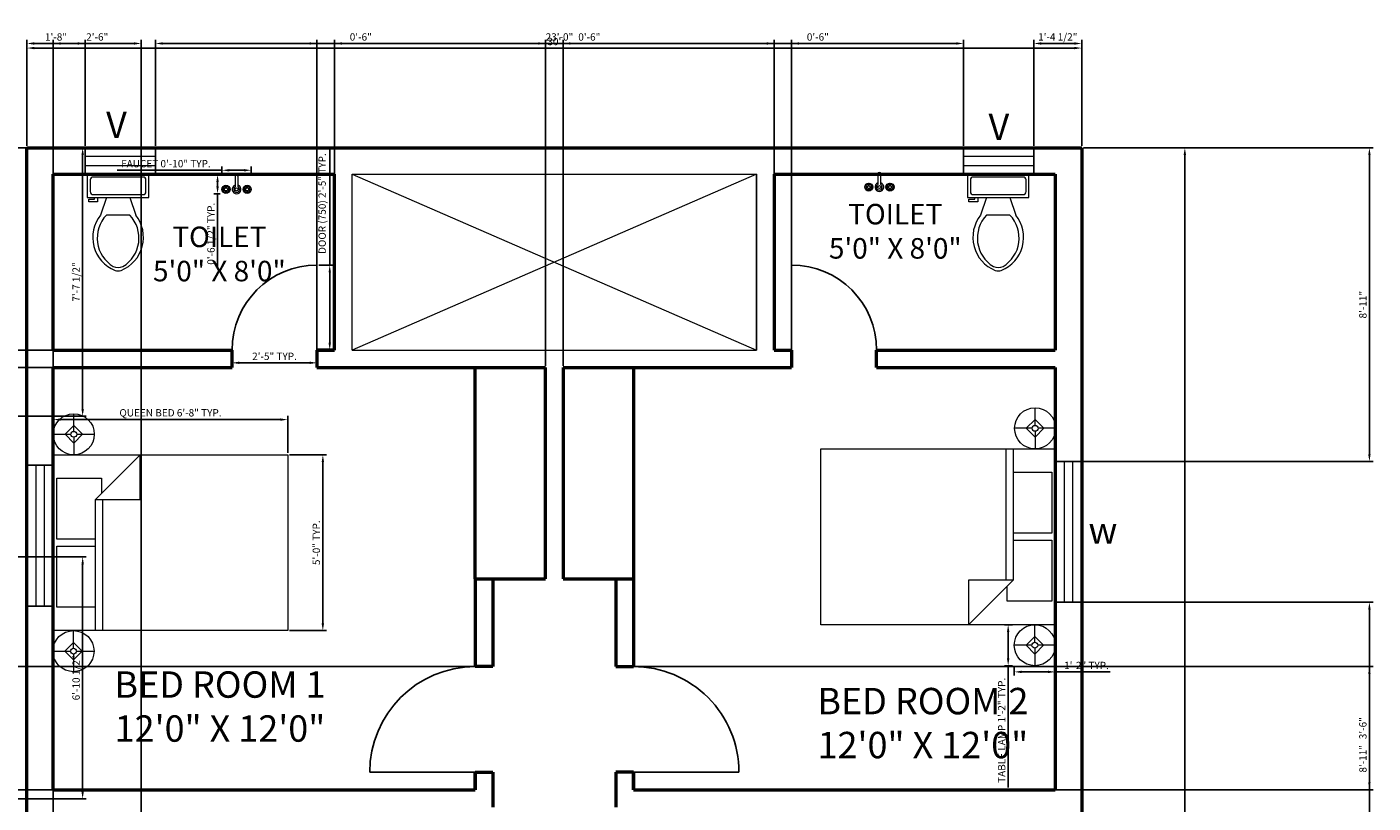
# Model space of a CAD drawing. Units: inches. Extents: x 3688 to 4628, y 1593 to 2337.
# Tile 7 of 7: x 4168 to 4628, y 2072 to 2337. Entities that reach past the tile are written whole.
import ezdxf

# ---------------------------------------------------------------- set-up
doc = ezdxf.new("R2010")
doc.units = ezdxf.units.IN
for name, color, linetype, lineweight in [('A-ANNO-DIMS', 2, 'Continuous', 18), ('A-ANNO-TEXT', 7, 'Continuous', 18), ('A-AREA-IDEN', 7, 'Continuous', 25), ('A-DOOR', 4, 'Continuous', 25), ('A-FLOR-FIXT', 8, 'Continuous', 18), ('A-FLOR-SHFT', 8, 'Continuous', 18), ('A-FURN', 8, 'Continuous', 18), ('A-GLAZ', 4, 'Continuous', 25), ('A-WALL', 7, 'Continuous', 50)]:
    doc.layers.add(name, color=color, linetype=linetype, lineweight=lineweight)
doc.styles.get("Standard").update_dxf_attribs({"font": 'arial.ttf'})
doc.dimstyles.new('ISO-25', dxfattribs={"dimtxt": 2.5, "dimasz": 2.5, "dimexe": 1.25, "dimexo": 0.625, "dimtad": 1, "dimdec": 0, "dimlunit": 3, "dimtxsty": 'Standard', "dimcen": 2.5, "dimadec": 0, "dimazin": 0, "dimtfac": 1, "dimtdec": 0, "dimtmove": 0, "dimatfit": 3, "dimfxl": 1, "dimarcsym": 0})

# ---------------------------------------------------------------- blocks, each defined once
blk = doc.blocks.new('Bed - Queen')
for p, q in [((0, -80.00003), (0, 0)), ((0, 0), (59.99999, 0)), ((59.99999, 0), (59.99999, -80.00003)), ((7.99999, -1.2), (28.79998, -1.2)), ((7.99999, -14.4), (7.99999, -1.2)), ((28.79998, -1.2), (28.79998, -14.4)), ((31.19999, -1.2), (51.99999, -1.2)), ((31.19999, -14.4), (31.19999, -1.2)), ((51.99999, -1.2), (51.99999, -16.4)), ((0, -14.4), (44.8, -14.4)), ((44.8, -16.8), (0, -16.8)), ((59.99999, -29.6), (44.8, -14.4)), ((44.8, -14.4), (44.8, -29.6)), ((51.99999, -16.4), (46.79936, -16.4)), ((44.8, -29.6), (59.99999, -29.6)), ((59.99999, -80.00003), (0, -80.00003))]:
    blk.add_line(p, q)
blk = doc.blocks.new('Lamp - Table')
for p, q in [((0, 7), (0, 1)), ((-1, 0), (-7, 0)), ((0, 3), (-3, 0)), ((-3, 0), (0, -3)), ((3, 0), (0, 3)), ((0, -3), (3, 0)), ((1, 0), (7, 0)), ((0, -1), (0, -7))]:
    blk.add_line(p, q)
for radius in [7, 1]:
    blk.add_circle((0, 0), radius)
blk = doc.blocks.new('Toilet - top')
for p, q in [((9.5, -6), (9.5, -2)), ((-10, -8.5), (-8, -8.5)), ((-10, -9.5), (-10, -8.5)), ((-8, -8.5), (-8, -8)), ((-7, -8), (-7, -9.5)), ((-4, -8), (-6, -14)), ((4, -8), (6, -14)), ((-7, -9.5), (-10, -9.5)), ((4, -14), (-4, -14))]:
    blk.add_line(p, q)
blk.add_lwpolyline([(10.5, -8), (10.5, 0), (-10.5, 0), (-10.5, -8)], close=True)
for points in [[(-9.5, -2), (-9.5, -6)], [(8.5, -1), (-8.5, -1)], [(-8.5, -7), (8.5, -7)]]:
    blk.add_lwpolyline(points)
for centre, radius, start, end in [((-8.62, -1.88), 0.884, 81.8699, 188.1301), ((8.62, -1.88), 0.884, 351.8699, 98.1301), ((-8.62, -6.12), 0.884, 171.8699, 278.1301), ((8.62, -6.12), 0.884, 261.8699, 8.1301), ((3.52, -21.58), 12.17, 141.4691, 247.9714), ((4.2, -21.82), 11.33, 136.3677, 238.9468), ((-3.52, -21.58), 12.17, 292.0284, 38.5307), ((-4.2, -21.82), 11.33, 301.053, 43.6321), ((0, -27.88), 4, 245.7318, 294.2682), ((0, -29), 4, 254.8605, 285.1395)]:
    blk.add_arc(centre, radius, start, end)
blk = doc.blocks.new('Faucet - Bathroom top')
for p, q in [((-4.107, 0.125), (-4.375, 0.125)), ((-3.75, 0.4788), (-3.75, 0.75)), ((-3.5, 0.482), (-3.5, 0.75)), ((-3.1461, 0.125), (-2.875, 0.125)), ((3.143, 0.125), (2.875, 0.125)), ((3.5, 0.4788), (3.5, 0.75)), ((3.75, 0.482), (3.75, 0.75)), ((4.1039, 0.125), (4.375, 0.125)), ((-4.1039, -0.125), (-4.375, -0.125)), ((-3.75, -0.4821), (-3.75, -0.75)), ((-3.5, -0.4789), (-3.5, -0.75)), ((-3.143, -0.125), (-2.875, -0.125)), ((-0.5, -0.8639), (-0.5, -4.5)), ((0.5, -4.5), (0.5, -0.8631)), ((3.1461, -0.125), (2.875, -0.125)), ((3.5, -0.4821), (3.5, -0.75)), ((3.75, -0.4789), (3.75, -0.75)), ((4.107, -0.125), (4.375, -0.125))]:
    blk.add_line(p, q)
for centre, radius in [((-3.625, 0), 1.375), ((-4.625, 0), 0.2795), ((-3.625, 0), 0.5), ((-3.625, 1), 0.2795), ((-2.625, 0), 0.2795), ((0, 0), 0.5), ((3.625, 0), 1.375), ((2.625, 0), 0.2795), ((3.625, 0), 0.5), ((3.625, 1), 0.2795), ((4.625, 0), 0.2795), ((-3.625, -1), 0.2795), ((3.625, -1), 0.2795)]:
    blk.add_circle(centre, radius)
for centre, radius, start, end in [((-3.625, 0), 1, 105.2407, 164.2093), ((-3.625, 0), 1, 16.44125, 74.07887), ((0, 0), 1.5, 289.6514, 250.3603), ((0, 0), 1, 300.3431, 239.7554), ((3.625, 0), 1, 106.12, 164.0884), ((3.625, 0), 1, 16.23422, 73.90469), ((-3.625, 0), 1, 196.2342, 253.9047), ((-3.625, 0), 1, 286.12, 344.0884), ((0, -4.5), 0.5, 180, 0), ((3.625, 0), 1, 196.4413, 254.0789), ((3.625, 0), 1, 285.2407, 344.2093)]:
    blk.add_arc(centre, radius, start, end)
blk = doc.blocks.new('*D14')
at = {"layer": 'A-ANNO-DIMS', "color": 0, "lineweight": -2, "transparency": 16777216}
for p, q in [((4168.13, 2295.91), (4168.13, 2330.57)), ((4528.13, 2295.91), (4528.13, 2330.57)), ((4170.63, 2329.32), (4525.63, 2329.32))]:
    blk.add_line(p, q, dxfattribs=at)
at = {"layer": 'A-ANNO-DIMS', "color": 0, "transparency": 16777216}
for points in [[(4170.63, 2329.74), (4170.63, 2328.91), (4168.13, 2329.32)], [(4525.63, 2329.74), (4525.63, 2328.91), (4528.13, 2329.32)]]:
    blk.add_solid(points, dxfattribs=at)
at = {"layer": 'Defpoints', "color": 0, "transparency": 16777216}
for p in [(4528.13, 2329.32), (4168.13, 2295.28), (4528.13, 2295.28)]:
    blk.add_point(p, dxfattribs=at)
at = {"layer": 'A-ANNO-DIMS', "color": 0, "transparency": 16777216, "insert": (4348.13, 2331.23), "char_height": 2.5, "attachment_point": 5}
blk.add_mtext("30'", dxfattribs=at)
blk = doc.blocks.new('*D15')
at = {"layer": 'A-ANNO-DIMS', "color": 0, "lineweight": -2, "transparency": 16777216}
for p, q in [((4528.76, 2295.28), (4564.58, 2295.28)), ((4563.33, 2292.78), (4563.33, 1697.78)), ((4528.76, 1695.28), (4564.58, 1695.28))]:
    blk.add_line(p, q, dxfattribs=at)
at = {"layer": 'A-ANNO-DIMS', "color": 0, "transparency": 16777216}
for points in [[(4562.91, 2292.78), (4563.75, 2292.78), (4563.33, 2295.28)], [(4562.91, 1697.78), (4563.75, 1697.78), (4563.33, 1695.28)]]:
    blk.add_solid(points, dxfattribs=at)
at = {"layer": 'Defpoints', "color": 0, "transparency": 16777216}
for p in [(4528.13, 2295.28), (4528.13, 1695.28), (4563.33, 1695.28)]:
    blk.add_point(p, dxfattribs=at)
at = {"layer": 'A-ANNO-DIMS', "color": 0, "transparency": 16777216, "insert": (4561.43, 1995.28), "char_height": 2.5, "attachment_point": 5, "rotation": 90}
blk.add_mtext("50'", dxfattribs=at)
blk = doc.blocks.new('DOOR-900')
blk.add_line((0, 0), (0, 36))
blk.add_arc((0, 0), 36, 0, 90)
blk = doc.blocks.new('DOOR-750')
blk.add_line((29, 0), (29, 29))
blk.add_arc((29, 0), 29, 90, 180)
blk = doc.blocks.new('WIN-1200')
for p, q in [((0, 48), (0, 0)), ((9, 48), (0, 48)), ((9, 0), (9, 48)), ((0, 0), (9, 0))]:
    blk.add_line(p, q)
blk = doc.blocks.new('WIN-600')
for p, q in [((24, 9), (0, 9)), ((0, 9), (0, 0)), ((24, 0), (24, 9)), ((0, 0), (24, 0))]:
    blk.add_line(p, q)
blk = doc.blocks.new('*D31')
at = {"layer": 'A-ANNO-DIMS', "color": 0, "lineweight": -2, "transparency": 16777216}
for p, q in [((4271.48, 2255.28), (4271.48, 2294.72)), ((4267.76, 2255.28), (4272.73, 2255.28)), ((4271.48, 2228.78), (4271.48, 2252.78)), ((4267.76, 2226.28), (4272.73, 2226.28))]:
    blk.add_line(p, q, dxfattribs=at)
at = {"layer": 'A-ANNO-DIMS', "color": 0, "transparency": 16777216}
for points in [[(4271.07, 2252.78), (4271.9, 2252.78), (4271.48, 2255.28)], [(4271.07, 2228.78), (4271.9, 2228.78), (4271.48, 2226.28)]]:
    blk.add_solid(points, dxfattribs=at)
at = {"layer": 'Defpoints', "color": 0, "transparency": 16777216}
for p in [(4267.13, 2255.28), (4271.48, 2255.28), (4267.13, 2226.28)]:
    blk.add_point(p, dxfattribs=at)
at = {"layer": 'A-ANNO-DIMS', "color": 0, "transparency": 16777216, "insert": (4269.22, 2276.25), "char_height": 2.5, "attachment_point": 5, "rotation": 90}
blk.add_mtext('DOOR (750) 2\'-5" TYP.', dxfattribs=at)
blk = doc.blocks.new('*D32')
at = {"layer": 'A-ANNO-DIMS', "color": 0, "lineweight": -2, "transparency": 16777216}
for p, q in [((4238.13, 2225.66), (4238.13, 2220.68)), ((4267.13, 2225.66), (4267.13, 2220.68)), ((4240.63, 2221.93), (4264.63, 2221.93))]:
    blk.add_line(p, q, dxfattribs=at)
at = {"layer": 'A-ANNO-DIMS', "color": 0, "transparency": 16777216}
for points in [[(4240.63, 2222.35), (4240.63, 2221.52), (4238.13, 2221.93)], [(4264.63, 2222.35), (4264.63, 2221.52), (4267.13, 2221.93)]]:
    blk.add_solid(points, dxfattribs=at)
at = {"layer": 'Defpoints', "color": 0, "transparency": 16777216}
for p in [(4238.13, 2226.28), (4267.13, 2226.28), (4267.13, 2221.93)]:
    blk.add_point(p, dxfattribs=at)
at = {"layer": 'A-ANNO-DIMS', "color": 0, "transparency": 16777216, "insert": (4252.63, 2223.83), "char_height": 2.5, "attachment_point": 5}
blk.add_mtext('2\'-5" TYP.', dxfattribs=at)
blk = doc.blocks.new('*D33')
at = {"layer": 'A-ANNO-DIMS', "color": 0, "lineweight": -2, "transparency": 16777216}
for p, q in [((4177.13, 2191.18), (4177.13, 2203.8)), ((4254.63, 2202.55), (4179.63, 2202.55)), ((4257.13, 2191.18), (4257.13, 2203.8))]:
    blk.add_line(p, q, dxfattribs=at)
at = {"layer": 'A-ANNO-DIMS', "color": 0, "transparency": 16777216}
for points in [[(4179.63, 2202.97), (4179.63, 2202.14), (4177.13, 2202.55)], [(4254.63, 2202.97), (4254.63, 2202.14), (4257.13, 2202.55)]]:
    blk.add_solid(points, dxfattribs=at)
at = {"layer": 'Defpoints', "color": 0, "transparency": 16777216}
for p in [(4177.13, 2202.55), (4177.13, 2190.55), (4257.13, 2190.55)]:
    blk.add_point(p, dxfattribs=at)
at = {"layer": 'A-ANNO-DIMS', "color": 0, "transparency": 16777216, "insert": (4217.13, 2204.55), "char_height": 2.5, "attachment_point": 5}
blk.add_mtext('QUEEN BED 6\'-8" TYP.', dxfattribs=at)
blk = doc.blocks.new('*D34')
at = {"layer": 'A-ANNO-DIMS', "color": 0, "lineweight": -2, "transparency": 16777216}
for p, q in [((4257.76, 2190.55), (4270.38, 2190.55)), ((4269.13, 2133.05), (4269.13, 2188.05)), ((4257.76, 2130.55), (4270.38, 2130.55))]:
    blk.add_line(p, q, dxfattribs=at)
at = {"layer": 'A-ANNO-DIMS', "color": 0, "transparency": 16777216}
for points in [[(4268.72, 2188.05), (4269.55, 2188.05), (4269.13, 2190.55)], [(4268.72, 2133.05), (4269.55, 2133.05), (4269.13, 2130.55)]]:
    blk.add_solid(points, dxfattribs=at)
at = {"layer": 'Defpoints', "color": 0, "transparency": 16777216}
for p in [(4257.13, 2190.55), (4269.13, 2190.55), (4257.13, 2130.55)]:
    blk.add_point(p, dxfattribs=at)
at = {"layer": 'A-ANNO-DIMS', "color": 0, "transparency": 16777216, "insert": (4267.23, 2160.55), "char_height": 2.5, "attachment_point": 5, "rotation": 90}
blk.add_mtext('5\'-0" TYP.', dxfattribs=at)
blk = doc.blocks.new('*D35')
at = {"layer": 'A-ANNO-DIMS', "color": 0, "lineweight": -2, "transparency": 16777216}
for p, q in [((4504.51, 2132.58), (4501.78, 2132.58)), ((4503.03, 2130.08), (4503.03, 2121.08)), ((4504.51, 2118.58), (4501.78, 2118.58)), ((4503.03, 2118.58), (4503.03, 2077.01))]:
    blk.add_line(p, q, dxfattribs=at)
at = {"layer": 'A-ANNO-DIMS', "color": 0, "transparency": 16777216}
for points in [[(4502.62, 2130.08), (4503.45, 2130.08), (4503.03, 2132.58)], [(4502.62, 2121.08), (4503.45, 2121.08), (4503.03, 2118.58)]]:
    blk.add_solid(points, dxfattribs=at)
at = {"layer": 'Defpoints', "color": 0, "transparency": 16777216}
for p in [(4505.13, 2132.58), (4503.03, 2118.58), (4505.13, 2118.58)]:
    blk.add_point(p, dxfattribs=at)
at = {"layer": 'A-ANNO-DIMS', "color": 0, "transparency": 16777216, "insert": (4501.15, 2096.55), "char_height": 2.5, "attachment_point": 5, "rotation": 90}
blk.add_mtext('TABLE LAMP 1\'-2" TYP.', dxfattribs=at)
blk = doc.blocks.new('*D36')
at = {"layer": 'A-ANNO-DIMS', "color": 0, "lineweight": -2, "transparency": 16777216}
for p, q in [((4505.13, 2117.96), (4505.13, 2115.23)), ((4507.63, 2116.48), (4516.63, 2116.48)), ((4519.13, 2117.96), (4519.13, 2115.23)), ((4519.13, 2116.48), (4537.89, 2116.48))]:
    blk.add_line(p, q, dxfattribs=at)
at = {"layer": 'A-ANNO-DIMS', "color": 0, "transparency": 16777216}
for points in [[(4507.63, 2116.9), (4507.63, 2116.07), (4505.13, 2116.48)], [(4516.63, 2116.9), (4516.63, 2116.07), (4519.13, 2116.48)]]:
    blk.add_solid(points, dxfattribs=at)
at = {"layer": 'Defpoints', "color": 0, "transparency": 16777216}
for p in [(4505.13, 2118.58), (4519.13, 2118.58), (4519.13, 2116.48)]:
    blk.add_point(p, dxfattribs=at)
at = {"layer": 'A-ANNO-DIMS', "color": 0, "transparency": 16777216, "insert": (4529.76, 2118.36), "char_height": 2.5, "attachment_point": 5}
blk.add_mtext('1\'-2" TYP.', dxfattribs=at)
blk = doc.blocks.new('*D39')
at = {"layer": 'A-ANNO-DIMS', "color": 0, "lineweight": -2, "transparency": 16777216}
for p, q in [((4234.7, 2286.75), (4234.7, 2288.88)), ((4244.7, 2286.75), (4244.7, 2288.88)), ((4234.7, 2287.63), (4198.97, 2287.63)), ((4242.2, 2287.63), (4237.2, 2287.63))]:
    blk.add_line(p, q, dxfattribs=at)
at = {"layer": 'A-ANNO-DIMS', "color": 0, "transparency": 16777216}
for points in [[(4237.2, 2288.04), (4237.2, 2287.21), (4234.7, 2287.63)], [(4242.2, 2288.04), (4242.2, 2287.21), (4244.7, 2287.63)]]:
    blk.add_solid(points, dxfattribs=at)
at = {"layer": 'Defpoints', "color": 0, "transparency": 16777216}
for p in [(4234.7, 2287.63), (4234.7, 2286.13), (4244.7, 2286.13)]:
    blk.add_point(p, dxfattribs=at)
at = {"layer": 'A-ANNO-DIMS', "color": 0, "transparency": 16777216, "insert": (4215.58, 2289.54), "char_height": 2.5, "attachment_point": 5}
blk.add_mtext('FAUCET 0\'-10" TYP.', dxfattribs=at)
blk = doc.blocks.new('*D40')
at = {"layer": 'A-ANNO-DIMS', "color": 0, "lineweight": -2, "transparency": 16777216}
for p, q in [((4234.07, 2286.13), (4231.95, 2286.13)), ((4233.2, 2283.63), (4233.2, 2282.13)), ((4234.07, 2279.63), (4231.95, 2279.63)), ((4233.2, 2279.63), (4233.2, 2254.81))]:
    blk.add_line(p, q, dxfattribs=at)
at = {"layer": 'A-ANNO-DIMS', "color": 0, "transparency": 16777216}
for points in [[(4232.78, 2283.63), (4233.61, 2283.63), (4233.2, 2286.13)], [(4232.78, 2282.13), (4233.61, 2282.13), (4233.2, 2279.63)]]:
    blk.add_solid(points, dxfattribs=at)
at = {"layer": 'Defpoints', "color": 0, "transparency": 16777216}
for p in [(4234.7, 2286.13), (4233.2, 2279.63), (4234.7, 2279.63)]:
    blk.add_point(p, dxfattribs=at)
at = {"layer": 'A-ANNO-DIMS', "color": 0, "transparency": 16777216, "insert": (4231.28, 2265.97), "char_height": 2.5, "attachment_point": 5, "rotation": 90}
blk.add_mtext('0\'-6 1/2" TYP.', dxfattribs=at)
blk = doc.blocks.new('*D57')
at = {"layer": 'A-ANNO-DIMS', "color": 0, "lineweight": -2, "transparency": 16777216}
for p, q in [((4090.25, 2295.32), (4188.4, 2295.32)), ((4187.15, 2292.82), (4187.15, 2206.19)), ((4090.25, 2203.69), (4188.4, 2203.69))]:
    blk.add_line(p, q, dxfattribs=at)
at = {"layer": 'A-ANNO-DIMS', "color": 0, "transparency": 16777216}
for points in [[(4186.74, 2292.82), (4187.57, 2292.82), (4187.15, 2295.32)], [(4186.74, 2206.19), (4187.57, 2206.19), (4187.15, 2203.69)]]:
    blk.add_solid(points, dxfattribs=at)
at = {"layer": 'Defpoints', "color": 0, "transparency": 16777216}
for p in [(4089.62, 2295.32), (4089.62, 2203.69), (4187.15, 2203.69)]:
    blk.add_point(p, dxfattribs=at)
at = {"layer": 'A-ANNO-DIMS', "color": 0, "transparency": 16777216, "insert": (4185.24, 2249.51), "char_height": 2.5, "attachment_point": 5, "rotation": 90}
blk.add_mtext('7\'-7 1/2"', dxfattribs=at)
blk = doc.blocks.new('*D58')
at = {"layer": 'A-ANNO-DIMS', "color": 0, "lineweight": -2, "transparency": 16777216}
for p, q in [((4090.25, 2155.69), (4188.4, 2155.69)), ((4187.15, 2153.19), (4187.15, 2075.67)), ((4090.25, 2073.17), (4188.4, 2073.17))]:
    blk.add_line(p, q, dxfattribs=at)
at = {"layer": 'A-ANNO-DIMS', "color": 0, "transparency": 16777216}
for points in [[(4186.74, 2153.19), (4187.57, 2153.19), (4187.15, 2155.69)], [(4186.74, 2075.67), (4187.57, 2075.67), (4187.15, 2073.17)]]:
    blk.add_solid(points, dxfattribs=at)
at = {"layer": 'Defpoints', "color": 0, "transparency": 16777216}
for p in [(4089.62, 2155.69), (4089.62, 2073.17), (4187.15, 2073.17)]:
    blk.add_point(p, dxfattribs=at)
at = {"layer": 'A-ANNO-DIMS', "color": 0, "transparency": 16777216, "insert": (4185.24, 2114.43), "char_height": 2.5, "attachment_point": 5, "rotation": 90}
blk.add_mtext('6\'-10 1/2"', dxfattribs=at)
blk = doc.blocks.new('*D85')
at = {"layer": 'A-ANNO-DIMS', "color": 0, "lineweight": -2, "transparency": 16777216}
for p, q in [((4528.76, 2295.28), (4627.58, 2295.28)), ((4626.33, 2292.78), (4626.33, 2190.76)), ((4528.76, 2188.26), (4627.58, 2188.26))]:
    blk.add_line(p, q, dxfattribs=at)
at = {"layer": 'A-ANNO-DIMS', "color": 0, "transparency": 16777216}
for points in [[(4625.91, 2292.78), (4626.74, 2292.78), (4626.33, 2295.28)], [(4625.91, 2190.76), (4626.74, 2190.76), (4626.33, 2188.26)]]:
    blk.add_solid(points, dxfattribs=at)
at = {"layer": 'Defpoints', "color": 0, "transparency": 16777216}
for p in [(4528.13, 2295.28), (4528.13, 2188.26), (4626.33, 2188.26)]:
    blk.add_point(p, dxfattribs=at)
at = {"layer": 'A-ANNO-DIMS', "color": 0, "transparency": 16777216, "insert": (4624.43, 2241.77), "char_height": 2.5, "attachment_point": 5, "rotation": 90}
blk.add_mtext('8\'-11"', dxfattribs=at)
blk = doc.blocks.new('*D86')
at = {"layer": 'A-ANNO-DIMS', "color": 0, "lineweight": -2, "transparency": 16777216}
for p, q in [((4528.76, 2140.26), (4627.58, 2140.26)), ((4626.33, 2137.76), (4626.33, 2035.89)), ((4528.76, 2033.39), (4627.58, 2033.39))]:
    blk.add_line(p, q, dxfattribs=at)
at = {"layer": 'A-ANNO-DIMS', "color": 0, "transparency": 16777216}
for points in [[(4625.91, 2137.76), (4626.74, 2137.76), (4626.33, 2140.26)], [(4625.91, 2035.89), (4626.74, 2035.89), (4626.33, 2033.39)]]:
    blk.add_solid(points, dxfattribs=at)
at = {"layer": 'Defpoints', "color": 0, "transparency": 16777216}
for p in [(4528.13, 2140.26), (4528.13, 2033.39), (4626.33, 2033.39)]:
    blk.add_point(p, dxfattribs=at)
at = {"layer": 'A-ANNO-DIMS', "color": 0, "transparency": 16777216, "insert": (4624.43, 2086.83), "char_height": 2.5, "attachment_point": 5, "rotation": 90}
blk.add_mtext('8\'-11"', dxfattribs=at)
blk = doc.blocks.new('*D89')
at = {"layer": 'A-ANNO-DIMS', "color": 0, "lineweight": -2, "transparency": 16777216}
for p, q in [((4168.13, 2295.91), (4168.13, 2332.13)), ((4170.63, 2330.88), (4185.49, 2330.88)), ((4187.99, 2295.91), (4187.99, 2332.13))]:
    blk.add_line(p, q, dxfattribs=at)
at = {"layer": 'A-ANNO-DIMS', "color": 0, "transparency": 16777216}
for points in [[(4170.63, 2331.3), (4170.63, 2330.47), (4168.13, 2330.88)], [(4185.49, 2331.3), (4185.49, 2330.47), (4187.99, 2330.88)]]:
    blk.add_solid(points, dxfattribs=at)
at = {"layer": 'Defpoints', "color": 0, "transparency": 16777216}
for p in [(4187.99, 2330.88), (4168.13, 2295.28), (4187.99, 2295.28)]:
    blk.add_point(p, dxfattribs=at)
at = {"layer": 'A-ANNO-DIMS', "color": 0, "transparency": 16777216, "insert": (4178.06, 2332.78), "char_height": 2.5, "attachment_point": 5}
blk.add_mtext('1\'-8"', dxfattribs=at)
blk = doc.blocks.new('*D90')
at = {"layer": 'A-ANNO-DIMS', "color": 0, "lineweight": -2, "transparency": 16777216}
for p, q in [((4211.99, 2295.91), (4211.99, 2332.13)), ((4214.49, 2330.88), (4485.3, 2330.88)), ((4487.8, 2295.91), (4487.8, 2332.13))]:
    blk.add_line(p, q, dxfattribs=at)
at = {"layer": 'A-ANNO-DIMS', "color": 0, "transparency": 16777216}
for points in [[(4214.49, 2331.3), (4214.49, 2330.47), (4211.99, 2330.88)], [(4485.3, 2331.3), (4485.3, 2330.47), (4487.8, 2330.88)]]:
    blk.add_solid(points, dxfattribs=at)
at = {"layer": 'Defpoints', "color": 0, "transparency": 16777216}
for p in [(4487.8, 2330.88), (4211.99, 2295.28), (4487.8, 2295.28)]:
    blk.add_point(p, dxfattribs=at)
at = {"layer": 'A-ANNO-DIMS', "color": 0, "transparency": 16777216, "insert": (4349.89, 2332.79), "char_height": 2.5, "attachment_point": 5}
blk.add_mtext('23\'-0"', dxfattribs=at)
blk = doc.blocks.new('*D91')
at = {"layer": 'A-ANNO-DIMS', "color": 0, "lineweight": -2, "transparency": 16777216}
for p, q in [((4511.8, 2295.91), (4511.8, 2332.13)), ((4514.3, 2330.88), (4525.63, 2330.88)), ((4528.13, 2295.91), (4528.13, 2332.13))]:
    blk.add_line(p, q, dxfattribs=at)
at = {"layer": 'A-ANNO-DIMS', "color": 0, "transparency": 16777216}
for points in [[(4514.3, 2331.3), (4514.3, 2330.47), (4511.8, 2330.88)], [(4525.63, 2331.3), (4525.63, 2330.47), (4528.13, 2330.88)]]:
    blk.add_solid(points, dxfattribs=at)
at = {"layer": 'Defpoints', "color": 0, "transparency": 16777216}
for p in [(4528.13, 2330.88), (4511.8, 2295.28), (4528.13, 2295.28)]:
    blk.add_point(p, dxfattribs=at)
at = {"layer": 'A-ANNO-DIMS', "color": 0, "transparency": 16777216, "insert": (4519.97, 2332.8), "char_height": 2.5, "attachment_point": 5}
blk.add_mtext('1\'-4 1/2"', dxfattribs=at)
blk = doc.blocks.new('*D92')
at = {"layer": 'A-ANNO-DIMS', "color": 0, "lineweight": -2, "transparency": 16777216}
for p, q in [((4264.63, 2330.88), (4262.13, 2330.88)), ((4267.13, 2226.91), (4267.13, 2332.13)), ((4267.13, 2330.88), (4273.13, 2330.88)), ((4273.13, 2226.91), (4273.13, 2332.13)), ((4275.63, 2330.88), (4286.03, 2330.88))]:
    blk.add_line(p, q, dxfattribs=at)
at = {"layer": 'A-ANNO-DIMS', "color": 0, "transparency": 16777216}
for points in [[(4264.63, 2331.3), (4264.63, 2330.47), (4267.13, 2330.88)], [(4275.63, 2331.3), (4275.63, 2330.47), (4273.13, 2330.88)]]:
    blk.add_solid(points, dxfattribs=at)
at = {"layer": 'Defpoints', "color": 0, "transparency": 16777216}
for p in [(4273.13, 2330.88), (4267.13, 2226.28), (4273.13, 2226.28)]:
    blk.add_point(p, dxfattribs=at)
at = {"layer": 'A-ANNO-DIMS', "color": 0, "transparency": 16777216, "insert": (4282.08, 2332.78), "char_height": 2.5, "attachment_point": 5}
blk.add_mtext('0\'-6"', dxfattribs=at)
blk = doc.blocks.new('*D93')
at = {"layer": 'A-ANNO-DIMS', "color": 0, "lineweight": -2, "transparency": 16777216}
for p, q in [((4420.63, 2330.88), (4418.13, 2330.88)), ((4423.13, 2226.91), (4423.13, 2332.13)), ((4423.13, 2330.88), (4429.13, 2330.88)), ((4429.13, 2226.91), (4429.13, 2332.13)), ((4431.63, 2330.88), (4442.03, 2330.88))]:
    blk.add_line(p, q, dxfattribs=at)
at = {"layer": 'A-ANNO-DIMS', "color": 0, "transparency": 16777216}
for points in [[(4420.63, 2331.3), (4420.63, 2330.47), (4423.13, 2330.88)], [(4431.63, 2331.3), (4431.63, 2330.47), (4429.13, 2330.88)]]:
    blk.add_solid(points, dxfattribs=at)
at = {"layer": 'Defpoints', "color": 0, "transparency": 16777216}
for p in [(4429.13, 2330.88), (4423.13, 2226.28), (4429.13, 2226.28)]:
    blk.add_point(p, dxfattribs=at)
at = {"layer": 'A-ANNO-DIMS', "color": 0, "transparency": 16777216, "insert": (4438.08, 2332.78), "char_height": 2.5, "attachment_point": 5}
blk.add_mtext('0\'-6"', dxfattribs=at)
blk = doc.blocks.new('*D94')
at = {"layer": 'A-ANNO-DIMS', "color": 0, "lineweight": -2, "transparency": 16777216}
for p, q in [((4056.49, 2228.78), (4056.49, 2231.28)), ((4237.51, 2226.28), (4055.24, 2226.28)), ((4056.49, 2226.28), (4056.49, 2220.28)), ((4237.51, 2220.28), (4055.24, 2220.28)), ((4056.49, 2217.78), (4056.49, 2207.39))]:
    blk.add_line(p, q, dxfattribs=at)
at = {"layer": 'A-ANNO-DIMS', "color": 0, "transparency": 16777216}
for points in [[(4056.07, 2228.78), (4056.9, 2228.78), (4056.49, 2226.28)], [(4056.07, 2217.78), (4056.9, 2217.78), (4056.49, 2220.28)]]:
    blk.add_solid(points, dxfattribs=at)
at = {"layer": 'Defpoints', "color": 0, "transparency": 16777216}
for p in [(4238.13, 2226.28), (4056.49, 2220.28), (4238.13, 2220.28)]:
    blk.add_point(p, dxfattribs=at)
at = {"layer": 'A-ANNO-DIMS', "color": 0, "transparency": 16777216, "insert": (4054.58, 2211.34), "char_height": 2.5, "attachment_point": 5, "rotation": 90}
blk.add_mtext('0\'-6"', dxfattribs=at)
blk = doc.blocks.new('*D95')
at = {"layer": 'A-ANNO-DIMS', "color": 0, "lineweight": -2, "transparency": 16777216}
for p, q in [((4342.63, 2330.88), (4340.13, 2330.88)), ((4345.13, 2220.91), (4345.13, 2332.13)), ((4345.13, 2330.88), (4351.13, 2330.88)), ((4351.13, 2220.91), (4351.13, 2332.13)), ((4353.63, 2330.88), (4364.03, 2330.88))]:
    blk.add_line(p, q, dxfattribs=at)
at = {"layer": 'A-ANNO-DIMS', "color": 0, "transparency": 16777216}
for points in [[(4342.63, 2331.3), (4342.63, 2330.47), (4345.13, 2330.88)], [(4353.63, 2331.3), (4353.63, 2330.47), (4351.13, 2330.88)]]:
    blk.add_solid(points, dxfattribs=at)
at = {"layer": 'Defpoints', "color": 0, "transparency": 16777216}
for p in [(4351.13, 2330.88), (4345.13, 2220.28), (4351.13, 2220.28)]:
    blk.add_point(p, dxfattribs=at)
at = {"layer": 'A-ANNO-DIMS', "color": 0, "transparency": 16777216, "insert": (4360.08, 2332.78), "char_height": 2.5, "attachment_point": 5}
blk.add_mtext('0\'-6"', dxfattribs=at)
blk = doc.blocks.new('*D96')
at = {"layer": 'A-ANNO-DIMS', "color": 0, "lineweight": -2, "transparency": 16777216}
for p, q in [((4320.51, 2118.28), (4055.24, 2118.28)), ((4056.49, 2115.78), (4056.49, 2078.78)), ((4320.51, 2076.28), (4055.24, 2076.28))]:
    blk.add_line(p, q, dxfattribs=at)
at = {"layer": 'A-ANNO-DIMS', "color": 0, "transparency": 16777216}
for points in [[(4056.07, 2115.78), (4056.9, 2115.78), (4056.49, 2118.28)], [(4056.07, 2078.78), (4056.9, 2078.78), (4056.49, 2076.28)]]:
    blk.add_solid(points, dxfattribs=at)
at = {"layer": 'Defpoints', "color": 0, "transparency": 16777216}
for p in [(4321.13, 2118.28), (4056.49, 2076.28), (4321.13, 2076.28)]:
    blk.add_point(p, dxfattribs=at)
at = {"layer": 'A-ANNO-DIMS', "color": 0, "transparency": 16777216, "insert": (4054.58, 2097.28), "char_height": 2.5, "attachment_point": 5, "rotation": 90}
blk.add_mtext('3\'-6"', dxfattribs=at)
blk = doc.blocks.new('*D97')
at = {"layer": 'A-ANNO-DIMS', "color": 0, "lineweight": -2, "transparency": 16777216}
for p, q in [((4375.76, 2118.28), (4627.58, 2118.28)), ((4626.33, 2115.78), (4626.33, 2078.78)), ((4375.76, 2076.28), (4627.58, 2076.28))]:
    blk.add_line(p, q, dxfattribs=at)
at = {"layer": 'A-ANNO-DIMS', "color": 0, "transparency": 16777216}
for points in [[(4625.91, 2115.78), (4626.74, 2115.78), (4626.33, 2118.28)], [(4625.91, 2078.78), (4626.74, 2078.78), (4626.33, 2076.28)]]:
    blk.add_solid(points, dxfattribs=at)
at = {"layer": 'Defpoints', "color": 0, "transparency": 16777216}
for p in [(4375.13, 2118.28), (4375.13, 2076.28), (4626.33, 2076.28)]:
    blk.add_point(p, dxfattribs=at)
at = {"layer": 'A-ANNO-DIMS', "color": 0, "transparency": 16777216, "insert": (4624.42, 2097.28), "char_height": 2.5, "attachment_point": 5, "rotation": 90}
blk.add_mtext('3\'-6"', dxfattribs=at)
blk = doc.blocks.new('*D98')
at = {"layer": 'A-ANNO-DIMS', "color": 0, "lineweight": -2, "transparency": 16777216}
for p, q in [((4177.13, 2010.91), (4177.13, 2332.13)), ((4179.63, 2330.88), (4204.63, 2330.88)), ((4207.13, 2010.91), (4207.13, 2332.13))]:
    blk.add_line(p, q, dxfattribs=at)
at = {"layer": 'A-ANNO-DIMS', "color": 0, "transparency": 16777216}
for points in [[(4179.63, 2331.3), (4179.63, 2330.47), (4177.13, 2330.88)], [(4204.63, 2331.3), (4204.63, 2330.47), (4207.13, 2330.88)]]:
    blk.add_solid(points, dxfattribs=at)
at = {"layer": 'Defpoints', "color": 0, "transparency": 16777216}
for p in [(4207.13, 2330.88), (4177.13, 2010.28), (4207.13, 2010.28)]:
    blk.add_point(p, dxfattribs=at)
at = {"layer": 'A-ANNO-DIMS', "color": 0, "transparency": 16777216, "insert": (4192.13, 2332.78), "char_height": 2.5, "attachment_point": 5}
blk.add_mtext('2\'-6"', dxfattribs=at)

msp = doc.modelspace()

# ---------------------------------------------------------------- linework, layer by layer
at = {"layer": 'A-DOOR'}
msp.add_line((4285.13, 2082.28), (4321.13, 2082.28), dxfattribs=at)
at = {"layer": 'A-FLOR-SHFT'}
for p, q in [((4279.13, 2226.28), (4279.13, 2286.28)), ((4279.13, 2286.28), (4417.13, 2286.28)), ((4279.13, 2286.28), (4417.13, 2226.28)), ((4417.13, 2286.28), (4279.13, 2226.28)), ((4417.13, 2286.28), (4417.13, 2226.28)), ((4417.13, 2226.28), (4417.13, 2286.28)), ((4279.13, 2226.28), (4417.13, 2226.28))]:
    msp.add_line(p, q, dxfattribs=at)
at = {"layer": 'A-FURN'}
for p, q in [((4211.99, 2292.28), (4187.99, 2292.28)), ((4187.99, 2289.28), (4211.99, 2289.28)), ((4511.8, 2292.28), (4487.8, 2292.28)), ((4487.8, 2289.28), (4511.8, 2289.28)), ((4171.13, 2186.96), (4171.13, 2138.96)), ((4174.13, 2138.96), (4174.13, 2186.96)), ((4522.13, 2188.26), (4522.13, 2140.26)), ((4525.13, 2140.26), (4525.13, 2188.26))]:
    msp.add_line(p, q, dxfattribs=at)
at = {"layer": 'A-WALL'}
for p, q in [((4168.13, 2295.28), (4528.13, 2295.28)), ((4168.13, 1695.28), (4168.13, 2295.28)), ((4528.13, 2295.28), (4528.13, 1695.28)), ((4177.13, 2286.28), (4273.13, 2286.28)), ((4177.13, 2226.28), (4177.13, 2286.28)), ((4273.13, 2226.28), (4273.13, 2286.28)), ((4423.13, 2286.28), (4423.13, 2226.28)), ((4423.13, 2286.28), (4519.13, 2286.28)), ((4519.13, 2286.28), (4519.13, 2226.28)), ((4177.13, 2226.28), (4238.13, 2226.28)), ((4238.13, 2220.28), (4238.13, 2226.28)), ((4273.13, 2226.28), (4267.13, 2226.28)), ((4267.13, 2226.28), (4267.13, 2220.28)), ((4267.13, 2226.28), (4273.13, 2226.28)), ((4423.13, 2226.28), (4429.13, 2226.28)), ((4423.13, 2226.28), (4429.13, 2226.28)), ((4429.13, 2226.28), (4429.13, 2220.28)), ((4458.13, 2220.28), (4458.13, 2226.28)), ((4458.13, 2226.28), (4519.13, 2226.28)), ((4177.13, 2220.28), (4238.13, 2220.28)), ((4177.13, 2076.28), (4177.13, 2220.28)), ((4267.13, 2220.28), (4345.13, 2220.28)), ((4321.13, 2148.28), (4321.13, 2220.28)), ((4345.13, 2148.28), (4345.13, 2220.28)), ((4351.13, 2220.28), (4351.13, 2148.28)), ((4351.13, 2220.28), (4429.13, 2220.28)), ((4375.13, 2220.28), (4375.13, 2148.28)), ((4458.13, 2220.28), (4519.13, 2220.28)), ((4519.13, 2220.28), (4519.13, 2076.28)), ((4321.13, 2148.28), (4345.13, 2148.28)), ((4321.13, 2148.28), (4321.13, 2118.28)), ((4327.13, 2148.28), (4327.13, 2118.28)), ((4351.13, 2148.28), (4375.13, 2148.28)), ((4369.13, 2148.28), (4369.13, 2118.28)), ((4375.13, 2148.28), (4375.13, 2118.28)), ((4327.13, 2118.28), (4321.13, 2118.28)), ((4369.13, 2118.28), (4375.13, 2118.28)), ((4321.13, 2076.28), (4321.13, 2082.28)), ((4321.13, 2082.28), (4327.13, 2082.28)), ((4321.13, 2082.28), (4321.13, 2076.28)), ((4327.13, 2082.28), (4327.13, 2070.28)), ((4375.13, 2082.28), (4369.13, 2082.28)), ((4369.13, 2082.28), (4369.13, 2070.28)), ((4375.13, 2076.28), (4375.13, 2082.28)), ((4375.13, 2082.28), (4375.13, 2076.28)), ((4177.13, 2076.28), (4321.13, 2076.28)), ((4375.13, 2076.28), (4519.13, 2076.28))]:
    msp.add_line(p, q, dxfattribs=at)

# ---------------------------------------------------------------- block references
at = {"layer": 'A-DOOR'}
msp.add_blockref('DOOR-750', (4238.13, 2226.28), dxfattribs=at)
at = {"layer": 'A-DOOR', "extrusion": (0, 0, -1), "zscale": -1}
msp.add_blockref('DOOR-750', (-4458.13, 2226.28), dxfattribs=at)
at = {"layer": 'A-DOOR', "rotation": 90}
msp.add_blockref('DOOR-900', (4321.13, 2082.28), dxfattribs=at)
at = {"layer": 'A-DOOR', "extrusion": (0, 0, -1), "zscale": -1, "rotation": 89.99999999999856}
msp.add_blockref('DOOR-900', (-4375.13, 2082.28), dxfattribs=at)
at = {"layer": 'A-FLOR-FIXT'}
for p in [(4199.25, 2286.32), (4499.64, 2286.32)]:
    msp.add_blockref('Toilet - top', p, dxfattribs=at)
at = {"layer": 'A-FLOR-FIXT', "rotation": 180}
for p in [(4239.7, 2281.13), (4459.07, 2281.89)]:
    msp.add_blockref('Faucet - Bathroom top', p, dxfattribs=at)
at = {"layer": 'A-FURN'}
for name, p, rotation in [('Lamp - Table', (4512.23, 2199.58), 270), ('Lamp - Table', (4184.13, 2197.55), 90), ('Bed - Queen', (4519.13, 2192.58), 270), ('Bed - Queen', (4177.13, 2130.55), 90), ('Lamp - Table', (4512.13, 2125.58), 270), ('Lamp - Table', (4184.03, 2123.55), 90)]:
    msp.add_blockref(name, p, dxfattribs=dict(at, rotation=rotation))
at = {"layer": 'A-GLAZ'}
for name, p in [('WIN-600', (4187.99, 2286.28)), ('WIN-600', (4487.8, 2286.28)), ('WIN-1200', (4168.13, 2138.96)), ('WIN-1200', (4519.13, 2140.26))]:
    msp.add_blockref(name, p, dxfattribs=at)

# ---------------------------------------------------------------- texts
at = {"layer": 'A-ANNO-TEXT', "char_height": 9, "attachment_point": 1}
for s, heights, insert in [('\\pxqc;V', [37.18], (4129.45, 2307.64)), ('\\pxqc;V', [37.18], (4430.62, 2306.93)), ('\\pxqc;w', [0], (4466.13, 2169.24))]:
    msp.add_mtext_dynamic_manual_height_columns(s, width=138.4723, gutter_width=12.5, heights=heights, dxfattribs=dict(at, insert=insert))
at = {"layer": 'A-AREA-IDEN', "attachment_point": 1}
for s, width, insert, char_height in [('\\pxqc;TOILET \\P5\'0" X 8\'0"', 61.3205, (4433.85, 2276.15), 7), ('\\pxqc;TOILET \\P5\'0" X 8\'0"', 61.3205, (4203.16, 2268.4), 7), ('\\pxqc;BED ROOM 1\\P12\'0" X 12\'0"', 105.0766, (4181.48, 2116.66), 9), ('\\pxqc;BED ROOM 2\\P12\'0" X 12\'0"', 105.0766, (4421.39, 2111.02), 9)]:
    msp.add_mtext_dynamic_manual_height_columns(s, width=width, gutter_width=12.5, heights=[0], dxfattribs=dict(at, insert=insert, char_height=char_height))

# ---------------------------------------------------------------- dimensions: what is measured, and where the dimension line sits
at = {"layer": 'A-ANNO-DIMS'}
for base, p1, p2, override, picture, middle in [((4187.99, 2330.88), (4168.13, 2295.28), (4187.99, 2295.28), {"dimdec": 1, "dimlfac": 1, "dimrnd": 0, "dimzin": 1, "dimdsep": 46, "dimlunit": 4, "dimfrac": 2}, '*D89', (4178.06, 2332.78)), ((4207.13, 2330.88), (4177.13, 2010.28), (4207.13, 2010.28), {"dimdec": 1, "dimlfac": 1, "dimrnd": 0, "dimzin": 1, "dimdsep": 46, "dimlunit": 4, "dimfrac": 2}, '*D98', (4192.13, 2332.78)), ((4487.8, 2330.88), (4211.99, 2295.28), (4487.8, 2295.28), {"dimdec": 1, "dimlfac": 1, "dimrnd": 0, "dimzin": 1, "dimdsep": 46, "dimlunit": 4, "dimfrac": 2}, '*D90', (4349.89, 2332.79)), ((4273.13, 2330.88), (4267.13, 2226.28), (4273.13, 2226.28), {"dimdec": 1, "dimlfac": 1, "dimrnd": 0, "dimzin": 1, "dimdsep": 46, "dimlunit": 4, "dimfrac": 2}, '*D92', (4282.08, 2332.78)), ((4351.13, 2330.88), (4345.13, 2220.28), (4351.13, 2220.28), {"dimdec": 1, "dimlfac": 1, "dimrnd": 0, "dimzin": 1, "dimdsep": 46, "dimlunit": 4, "dimfrac": 2}, '*D95', (4360.08, 2332.78)), ((4429.13, 2330.88), (4423.13, 2226.28), (4429.13, 2226.28), {"dimdec": 1, "dimlfac": 1, "dimrnd": 0, "dimzin": 1, "dimdsep": 46, "dimlunit": 4, "dimfrac": 2}, '*D93', (4438.08, 2332.78)), ((4528.13, 2330.88), (4511.8, 2295.28), (4528.13, 2295.28), {"dimdec": 1, "dimlfac": 1, "dimrnd": 0, "dimzin": 1, "dimdsep": 46, "dimlunit": 4, "dimfrac": 2}, '*D91', (4519.97, 2332.8)), ((4528.13, 2329.32), (4168.13, 2295.28), (4528.13, 2295.28), {"dimclrd": 0, "dimclre": 0, "dimclrt": 0}, '*D14', (4348.13, 2331.23))]:
    dim = msp.add_linear_dim(base=base, p1=p1, p2=p2, dimstyle='ISO-25', override=override, dxfattribs=at)
    dim.commit()
    dim.dimension.update_dxf_attribs({"geometry": picture, "text_midpoint": middle})
for base, p1, p2, override, picture, middle in [((4187.15, 2203.69), (4089.62, 2295.32), (4089.62, 2203.69), {"dimdec": 1, "dimlfac": 1, "dimrnd": 0, "dimzin": 1, "dimdsep": 46, "dimlunit": 4, "dimfrac": 2}, '*D57', (4185.24, 2249.51)), ((4563.33, 1695.28), (4528.13, 2295.28), (4528.13, 1695.28), {"dimclrd": 0, "dimclre": 0, "dimclrt": 0}, '*D15', (4561.43, 1995.28)), ((4626.33, 2188.26), (4528.13, 2295.28), (4528.13, 2188.26), {"dimdec": 1, "dimlfac": 1, "dimrnd": 0, "dimzin": 1, "dimdsep": 46, "dimlunit": 4, "dimfrac": 2}, '*D85', (4624.43, 2241.77)), ((4056.49, 2220.28), (4238.13, 2226.28), (4238.13, 2220.28), {"dimdec": 1, "dimlfac": 1, "dimrnd": 0, "dimzin": 1, "dimdsep": 46, "dimlunit": 4, "dimfrac": 2}, '*D94', (4054.58, 2211.34)), ((4187.15, 2073.17), (4089.62, 2155.69), (4089.62, 2073.17), {"dimdec": 1, "dimlfac": 1, "dimrnd": 0, "dimzin": 1, "dimdsep": 46, "dimlunit": 4, "dimfrac": 2}, '*D58', (4185.24, 2114.43)), ((4626.33, 2033.39), (4528.13, 2140.26), (4528.13, 2033.39), {"dimdec": 1, "dimlfac": 1, "dimrnd": 0, "dimzin": 1, "dimdsep": 46, "dimlunit": 4, "dimfrac": 2}, '*D86', (4624.43, 2086.83)), ((4056.49, 2076.28), (4321.13, 2118.28), (4321.13, 2076.28), {"dimdec": 1, "dimlfac": 1, "dimrnd": 0, "dimzin": 1, "dimdsep": 46, "dimlunit": 4, "dimfrac": 2}, '*D96', (4054.58, 2097.28)), ((4626.33, 2076.28), (4375.13, 2118.28), (4375.13, 2076.28), {"dimdec": 1, "dimlfac": 1, "dimrnd": 0, "dimzin": 1, "dimdsep": 46, "dimlunit": 4, "dimfrac": 2}, '*D97', (4624.42, 2097.28))]:
    dim = msp.add_linear_dim(base=base, p1=p1, p2=p2, angle=90, dimstyle='ISO-25', override=override, dxfattribs=at)
    dim.commit()
    dim.dimension.update_dxf_attribs({"geometry": picture, "text_midpoint": middle})
for base, p1, p2, angle, text, picture, middle in [((4234.7, 2287.63), (4244.7, 2286.13), (4234.7, 2286.13), 180, 'FAUCET <> TYP.', '*D39', (4215.58, 2289.54)), ((4271.48, 2255.28), (4267.13, 2226.28), (4267.13, 2255.28), 90, 'DOOR (750) <> TYP.', '*D31', (4269.22, 2276.25)), ((4233.2, 2279.63), (4234.7, 2286.13), (4234.7, 2279.63), 270, '<> TYP.', '*D40', (4231.28, 2265.97)), ((4177.13, 2202.55), (4257.13, 2190.55), (4177.13, 2190.55), 180, 'QUEEN BED <> TYP.', '*D33', (4217.13, 2204.55)), ((4269.13, 2190.55), (4257.13, 2130.55), (4257.13, 2190.55), 90, '<> TYP.', '*D34', (4267.23, 2160.55)), ((4503.03, 2118.58), (4505.13, 2132.58), (4505.13, 2118.58), 270, 'TABLE LAMP <> TYP.', '*D35', (4501.15, 2096.55))]:
    dim = msp.add_linear_dim(base=base, p1=p1, p2=p2, angle=angle, text=text, dimstyle='ISO-25', override={"dimdec": 1, "dimrnd": 0, "dimzin": 1, "dimlunit": 4, "dimfrac": 2}, dxfattribs=at)
    dim.commit()
    dim.dimension.update_dxf_attribs({"geometry": picture, "text_midpoint": middle})
for base, p1, p2, picture, middle in [((4267.13, 2221.93), (4238.13, 2226.28), (4267.13, 2226.28), '*D32', (4252.63, 2223.83)), ((4519.13, 2116.48), (4505.13, 2118.58), (4519.13, 2118.58), '*D36', (4529.76, 2118.36))]:
    dim = msp.add_linear_dim(base=base, p1=p1, p2=p2, text='<> TYP.', dimstyle='ISO-25', override={"dimdec": 1, "dimrnd": 0, "dimzin": 1, "dimlunit": 4, "dimfrac": 2}, dxfattribs=at)
    dim.commit()
    dim.dimension.update_dxf_attribs({"geometry": picture, "text_midpoint": middle})

doc.saveas('drawing.dxf')
